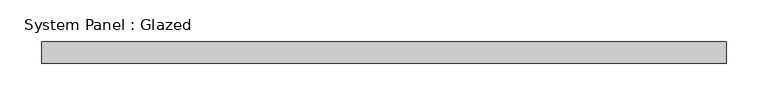
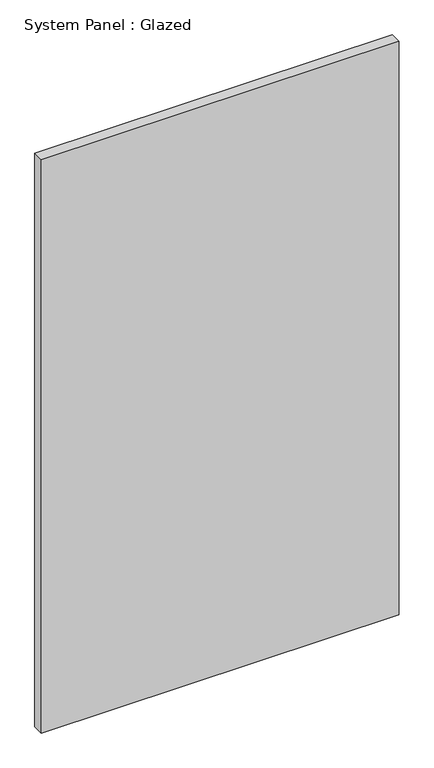
"""IFC4 building model written with IfcOpenShell, lengths in millimetres: plate geometry, System Panel : Glazed."""

from ifc_helpers import new_model, si_unit, origin, origin_with_axes, place, context, project, spatial, polyline, outline, extrude, source, transform, mapped, element, save


def system_panel_glazed_c96ed355(model_context):
    return source(origin(), model_context, "Body", "SweptSolid", [
        extrude(outline(polyline([(409.575, 19.05), (-409.575, 19.05), (-409.575, 44.45), (409.575, 44.45), (409.575, 19.05)])), origin_with_axes(), (0.0, 0.0, 1.0), 1386.786396),
    ])


if __name__ == "__main__":
    model = new_model("IFC4")
    model_context = context("Model", 3, world=origin())
    ifc_project = project(units=[si_unit("LENGTHUNIT", "METRE", prefix="MILLI")], contexts=[model_context])
    site = spatial("IfcSite", under=ifc_project)
    building = spatial("IfcBuilding", under=site)
    placement = place(None, origin())
    system_panel_glazed_shape = system_panel_glazed_c96ed355(model_context)
    element("IfcPlate", 1, ObjectType="System Panel : Glazed", at=placement, inside=building, context=model_context, shape_type="MappedRepresentation", body=[
        mapped(system_panel_glazed_shape, transform((0.0, 0.0, 0.0), x_axis=(1.0, 0.0, 0.0), y_axis=(0.0, 1.0, 0.0), z_axis=(0.0, 0.0, 1.0))),
    ])
    save(model, "model.ifc")

# Revit data of these elements
# Type "System Panel : Glazed"
#   Construction Type Id = "GSP4R"
#   Analytic Construction = "1/8 in Pilkington single glazing"
#   Visual Light Transmittance = 0.9
#   Solar Heat Gain Coefficient = 0.86
#   Heat Transfer Coefficient (U) = 1.18115 BTU/(h·ft²·°F)
#   Define Thermal Properties by = 1
# Element 1 (IfcPlate, "System Panel : Glazed")
#   Materials on its faces: "Glass"
# Materials
#   "Glass": class "Glass", colour RGB 0 128 192, transparency 0.75, Description = "Soda Lime Glass", Cost = 0
